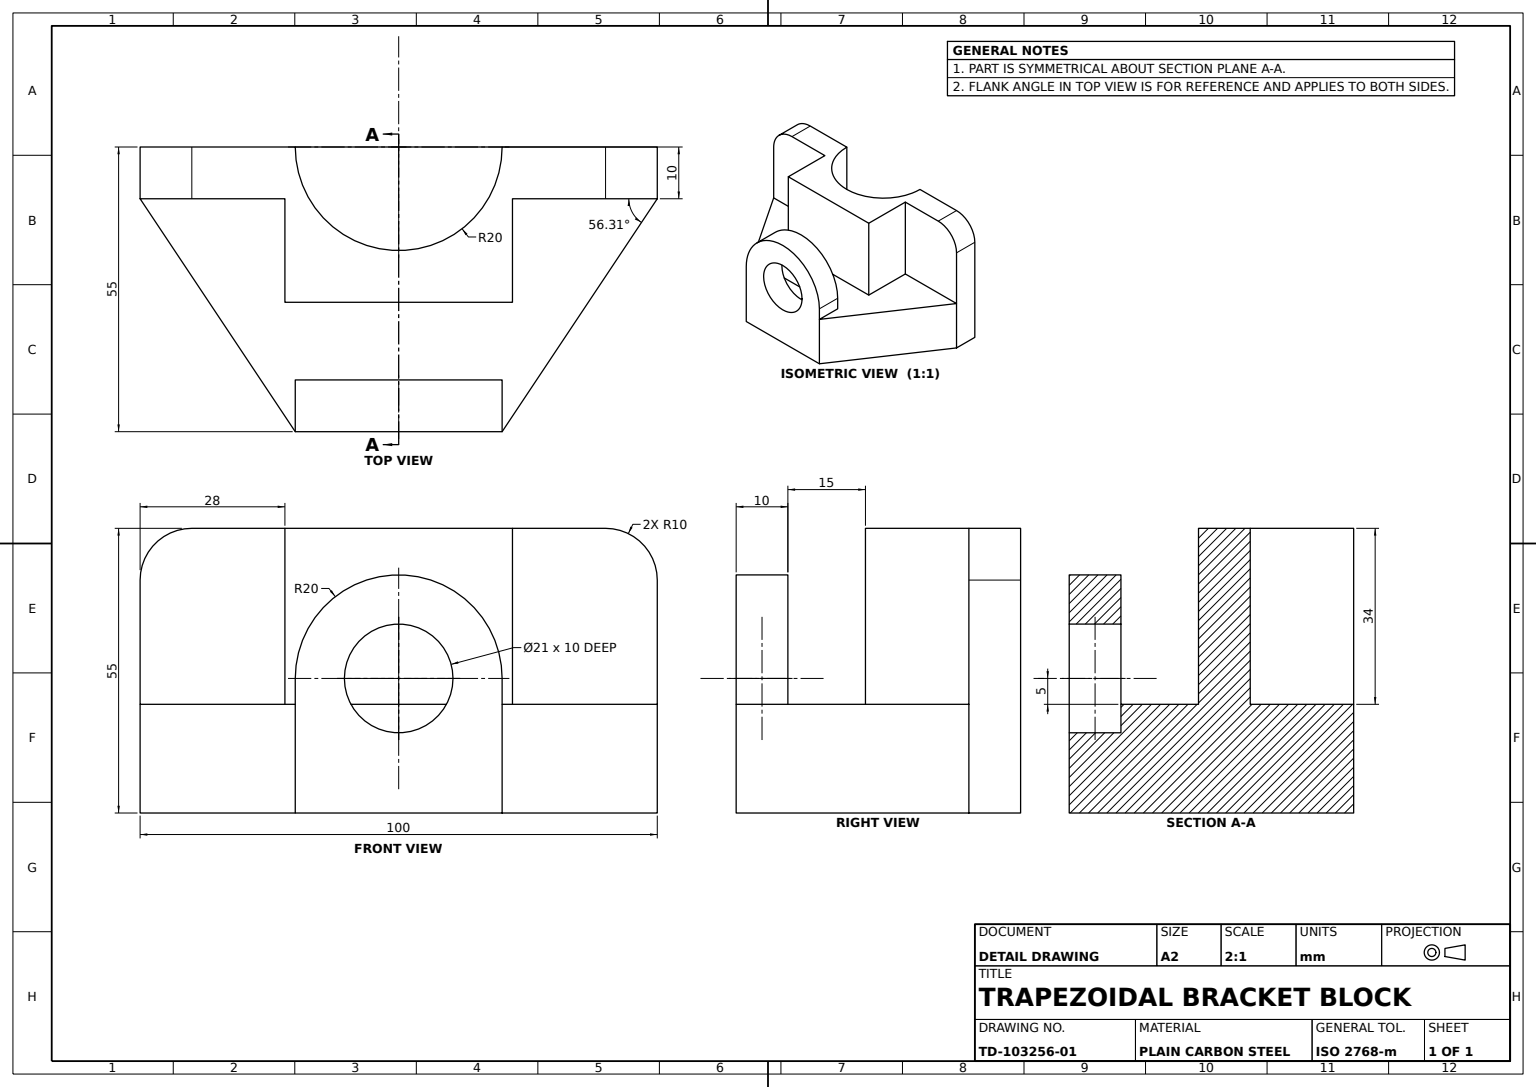
SolidWorks part; units mm, degrees
material "Plain Carbon Steel"
ref_plane "Front Plane" through (0, 0, 0) normal (0, 0, 1) x (1, 0, 0)
ref_plane "Top Plane" through (0, 0, 0) normal (0, 1, 0) x (1, 0, 0)
ref_plane "Right Plane" through (0, 0, 0) normal (1, 0, 0) x (0, 0, -1)
sketch "Base Profile Sketch" plane through (0, 0, 0) normal (0, 0, 1) x (1, 0, 0)
  line L0 (0, 0) -> (-50, 0)
  line L1 (0, 0) -> (50, 0)
  line L2 (-50, 0) -> (-50, -45)
  line L3 (50, 0) -> (50, -45)
  line L4 (-50, 0) -> (-40, 0)
  line L6 (50, 0) -> (40, 0)
  line L9 (-40, -55) -> (-22, -55)
  line L10 (-22, -55) -> (-22, -25)
  line L11 (40, -55) -> (22, -55)
  line L12 (22, -55) -> (22, -25)
  line L13 (22, -25) -> (-22, -25)
  arc A0 (-50, -45) -> (-40, -55) centre (-40, -45) ccw
  arc A1 (40, -55) -> (50, -45) centre (40, -45) ccw
  dimension "D1" = 20
  dimension "D2" = 20
  dimension "D3" = 10
  dimension "D4" = 28
  dimension "D5" = 50
  dimension "D6" = 30
  dimension "D7" = 55
extrude "Base Profile 10mm" add sketch "Base Profile Sketch" along normal blind 10 contours L11 A1 L3 L1 L0 L2 A0 L9 L10 L13 L12
sketch "Upper Block Sketch" plane through (0, -25, 0) normal (0, -1, 0) x (1, 0, 0)
  line L0 (-22, 10) -> (-22, 30)
  line L1 (22, 10) -> (22, 30)
  line L2 (22, 30) -> (-22, 30)
  line L4 (-22, 10) -> (-22, 0)
  line L5 (-22, 0) -> (22, 0)
  line L6 (22, 0) -> (22, 10)
  line L8 (22, 0) -> (-22, 0) construction
  dimension "D1" = 30
extrude "Upper Block 30mm" add sketch "Upper Block Sketch" along normal blind 30
sketch "Pad Sketch" plane through (0, -25, 0) normal (0, 1, 0) x (1, 0, 0)
  line L0 (-22, -10) -> (22, -10)
  line L1 (22, -10) -> (22, -30)
  line L2 (22, -30) -> (-22, -30)
  line L3 (-22, -30) -> (-22, -10)
extrude "Pad 4mm" add sketch "Pad Sketch" along normal blind 4
sketch "Profile Cut Sketch" plane through (0, -55, 0) normal (0, -1, 0) x (1, 0, 0)
  line L0 (-40, 0) -> (40, 0) construction
  line L1 (-20, 0) -> (20, 0)
  arc A0 (20, 0) -> (-20, 0) centre (0, 0) ccw
  dimension "D1" = 40
  dimension "D2" = 20
extrude "Profile Cut 34mm" cut sketch "Profile Cut Sketch" against normal blind 34
sketch "Side Wall Sketch" plane through (0, 0, 0) normal (0, 1, 0) x (1, 0, 0)
  line L0 (-50, -10) -> (-50, 0) construction
  line L1 (-50, -10) -> (50, -10) construction
  line L2 (0, -55) -> (20, -55)
  line L3 (20, -55) -> (50, -10)
  line L4 (50, -10) -> (50, 0) construction
  line L5 (50, -10) -> (-50, -10)
  line L6 (0, -55) -> (-20, -55)
  line L7 (-20, -55) -> (-50, -10)
  line L8 (-50, 0) -> (50, 0) construction
  dimension "D1" = 30
  dimension "D2" = 55
extrude "Side Wall 21mm" add sketch "Side Wall Sketch" against normal blind 21
sketch "Rail Sketch" plane through (0, -21, 0) normal (0, -1, 0) x (1, 0, 0)
  line L0 (-20, 55) -> (20, 55)
  line L1 (20, 55) -> (20, 45)
  line L2 (20, 45) -> (-20, 45)
  line L3 (-20, 45) -> (-20, 55)
  dimension "D1" = 15
extrude "Rail 5mm" add sketch "Rail Sketch" along normal blind 5
sketch "Lug Sketch" plane through (0, 0, 55) normal (0, 0, 1) x (1, 0, 0)
  line L0 (20, -26) -> (-20, -26) construction
  line L1 (-20, -26) -> (20, -26)
  arc A0 (-20, -26) -> (20, -26) centre (0, -26) ccw
  dimension "D1" = 40
  dimension "D2" = 20
extrude "Lug Boss 10mm" add sketch "Lug Sketch" against normal blind 10
sketch "Lug Hole Sketch Ø21" plane through (0, 0, 55) normal (0, 0, 1) x (1, 0, 0)
  circle A0 centre (0, -26) radius 10.5
  dimension "D1" = 21
  dimension "D2" = 21
extrude "Lug Hole Ø21" cut sketch "Lug Hole Sketch Ø21" against normal blind 10
